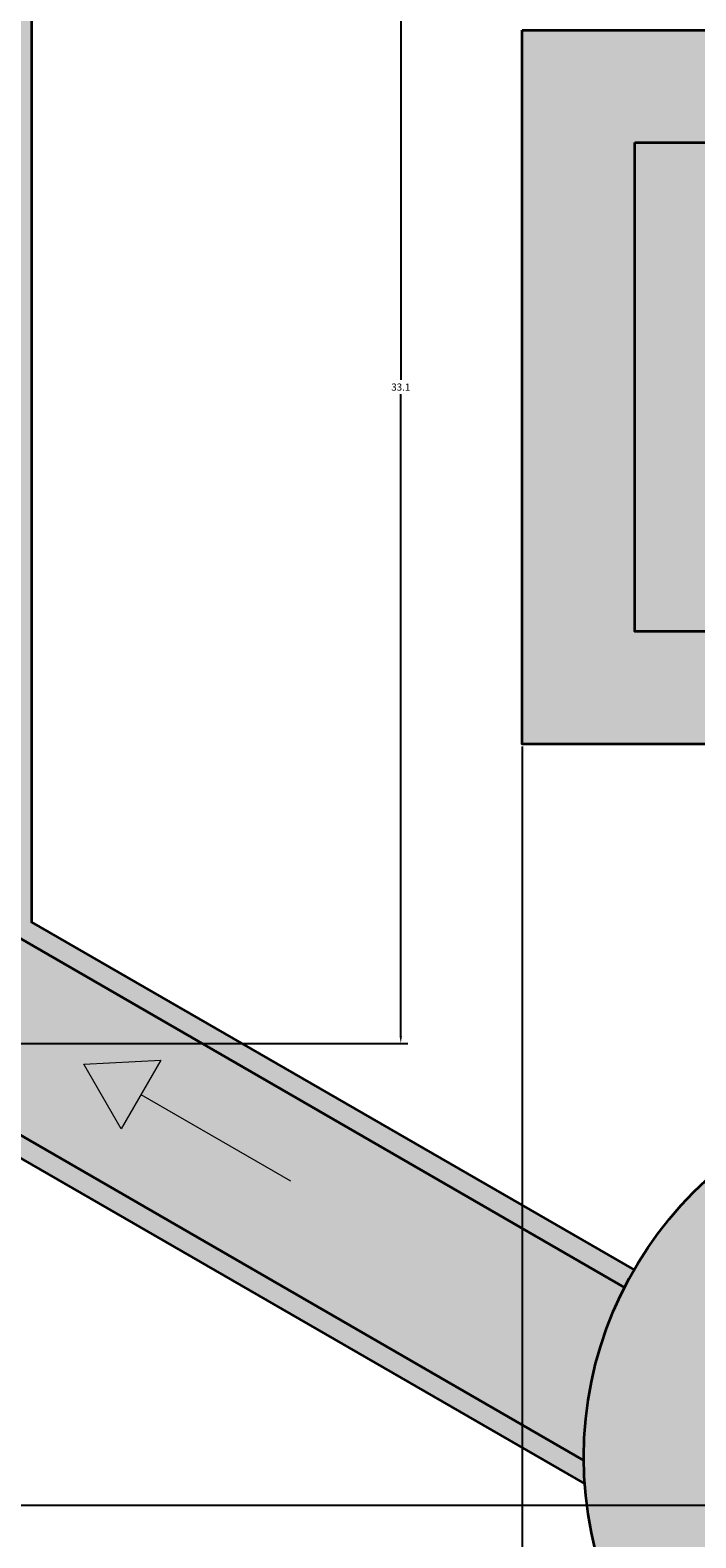
# Model space of a CAD drawing. Units: inches. Extents: x -1 to 292, y -3 to 199.
# Tile 43 of 52: x 220 to 237, y 43 to 81. Entities that reach past the tile are written whole.
import ezdxf

# ---------------------------------------------------------------- set-up
doc = ezdxf.new("R2010")
doc.units = ezdxf.units.IN
doc.header["$MEASUREMENT"] = 0
for name, color, linetype, lineweight in [('M-ANNO-SYMB', 1, 'Continuous', 18), ('M-DIMS', 2, 'Continuous', 18), ('M-EQPM', 7, 'Continuous', 35), ('M-PATT', 8, 'Continuous', 13)]:
    doc.layers.add(name, color=color, linetype=linetype, lineweight=lineweight)
doc.styles.get("Standard").update_dxf_attribs({"font": 'arial.ttf'})
doc.dimstyles.get("Standard").update_dxf_attribs({"dimtxt": 0.18, "dimasz": 0.18, "dimexe": 0.18, "dimexo": 0.0625, "dimgap": 0.09, "dimtad": 0, "dimtih": 1, "dimtoh": 1, "dimdec": 4, "dimzin": 0, "dimdsep": 46, "dimtxsty": 'Standard', "dimcen": 0.09, "dimadec": 0, "dimazin": 0, "dimtfac": 1, "dimtdec": 4, "dimtofl": 0, "dimtmove": 0, "dimatfit": 3, "dimfxl": 1, "dimtolj": 1, "dimtzin": 0, "dimarcsym": 0})

# ---------------------------------------------------------------- blocks, each defined once
blk = doc.blocks.new('FLOW-ARROW-WATER')
blk.add_line((223.29, 53.741), (227.063, 51.564))
blk.add_lwpolyline([(222.79, 52.875), (221.849, 54.506), (223.79, 54.608)], close=True)
blk = doc.blocks.new('*D10')
at = {"layer": 'Defpoints', "color": 0, "transparency": 16777216}
for p in [(169.176, 99.774), (169.176, 43.391), (292.04, 43.391)]:
    blk.add_point(p, dxfattribs=at)
at = {"layer": 'M-DIMS', "color": 0, "lineweight": -2, "transparency": 16777216}
for p, q in [((169.239, 99.774), (292.22, 99.774)), ((292.04, 99.594), (292.04, 71.764)), ((292.04, 43.571), (292.04, 71.4)), ((169.239, 43.391), (292.22, 43.391))]:
    blk.add_line(p, q, dxfattribs=at)
at = {"layer": 'M-DIMS', "color": 0, "transparency": 16777216}
for points in [[(292.01, 99.594), (292.07, 99.594), (292.04, 99.774)], [(292.01, 43.571), (292.07, 43.571), (292.04, 43.391)]]:
    blk.add_solid(points, dxfattribs=at)
at = {"layer": 'M-DIMS', "color": 0, "transparency": 16777216, "insert": (292.04, 71.582), "char_height": 0.18, "attachment_point": 5}
blk.add_mtext('\\A1;56.38', dxfattribs=at)
blk = doc.blocks.new('*D25')
at = {"layer": 'Defpoints', "color": 0, "transparency": 16777216}
for p in [(273.066, 88.419), (215.241, 88.13), (273.066, -2.71)]:
    blk.add_point(p, dxfattribs=at)
at = {"layer": 'M-DIMS', "color": 0, "lineweight": -2, "transparency": 16777216}
for p, q in [((273.066, 88.357), (273.066, -2.89)), ((215.241, 88.068), (215.241, -2.89)), ((215.421, -2.71), (243.76, -2.71)), ((272.886, -2.71), (244.547, -2.71))]:
    blk.add_line(p, q, dxfattribs=at)
at = {"layer": 'M-DIMS', "color": 0, "transparency": 16777216}
for points in [[(215.421, -2.68), (215.421, -2.74), (215.241, -2.71)], [(272.886, -2.68), (272.886, -2.74), (273.066, -2.71)]]:
    blk.add_solid(points, dxfattribs=at)
at = {"layer": 'M-DIMS', "color": 0, "transparency": 16777216, "insert": (244.153, -2.71), "char_height": 0.18, "attachment_point": 5}
blk.add_mtext('\\A1;57.83', dxfattribs=at)
blk = doc.blocks.new('*D26')
at = {"layer": 'Defpoints', "color": 0, "transparency": 16777216}
for p in [(215.241, 88.13), (215.241, 55.034), (229.841, 55.034)]:
    blk.add_point(p, dxfattribs=at)
at = {"layer": 'M-DIMS', "color": 0, "lineweight": -2, "transparency": 16777216}
for p, q in [((215.303, 88.13), (230.021, 88.13)), ((229.841, 87.95), (229.841, 71.764)), ((229.841, 55.214), (229.841, 71.4)), ((215.303, 55.034), (230.021, 55.034))]:
    blk.add_line(p, q, dxfattribs=at)
at = {"layer": 'M-DIMS', "color": 0, "transparency": 16777216}
for points in [[(229.811, 87.95), (229.871, 87.95), (229.841, 88.13)], [(229.811, 55.214), (229.871, 55.214), (229.841, 55.034)]]:
    blk.add_solid(points, dxfattribs=at)
at = {"layer": 'M-DIMS', "color": 0, "transparency": 16777216, "insert": (229.841, 71.582), "char_height": 0.18, "attachment_point": 5}
blk.add_mtext('\\A1;33.1', dxfattribs=at)
blk = doc.blocks.new('*D30')
at = {"layer": 'Defpoints', "color": 0, "transparency": 16777216}
for p in [(232.903, 62.582), (254.903, 62.582), (254.903, -2.71)]:
    blk.add_point(p, dxfattribs=at)
at = {"layer": 'M-DIMS', "color": 0, "lineweight": -2, "transparency": 16777216}
for p, q in [((232.903, 62.52), (232.903, -2.89)), ((254.903, 62.52), (254.903, -2.89)), ((233.083, -2.71), (243.684, -2.71)), ((254.723, -2.71), (244.123, -2.71))]:
    blk.add_line(p, q, dxfattribs=at)
at = {"layer": 'M-DIMS', "color": 0, "transparency": 16777216}
for points in [[(233.083, -2.68), (233.083, -2.74), (232.903, -2.71)], [(254.723, -2.68), (254.723, -2.74), (254.903, -2.71)]]:
    blk.add_solid(points, dxfattribs=at)
at = {"layer": 'M-DIMS', "color": 0, "transparency": 16777216, "insert": (243.903, -2.71), "char_height": 0.18, "attachment_point": 5}
blk.add_mtext('\\A1;22', dxfattribs=at)
blk = doc.blocks.new('*D36')
at = {"layer": 'Defpoints', "color": 0, "transparency": 16777216}
for p in [(234.455, 44.597), (253.352, 44.598)]:
    blk.add_point(p, dxfattribs=at)
at = {"layer": 'M-DIMS', "color": 0, "lineweight": -2, "transparency": 16777216}
for p, q in [((243.813, 44.598), (243.993, 44.598)), ((243.903, 44.508), (243.903, 44.688)), ((259.021, 44.598), (253.532, 44.598))]:
    blk.add_line(p, q, dxfattribs=at)
at = {"layer": 'M-DIMS', "color": 0, "transparency": 16777216}
blk.add_solid([(253.532, 44.628), (253.532, 44.568), (253.352, 44.598)], dxfattribs=at)
at = {"layer": 'M-DIMS', "color": 0, "transparency": 16777216, "insert": (259.582, 44.598), "char_height": 0.18, "attachment_point": 5}
blk.add_mtext('\\A1;∅18.897', dxfattribs=at)

msp = doc.modelspace()

# ---------------------------------------------------------------- hatches: boundary and pattern name
at = {"layer": 'M-PATT'}
h = msp.add_hatch(color=256, dxfattribs=at)
h.set_gradient(color1=(0, 255, 255), color2=(0, 255, 255), tint=1, name='CYLINDER')
h.paths.add_polyline_path([(256.8092, 99.5764), (256.4077, 99.3157), (253.7155, 100.87), (251.3221, 99.3157), (248.6299, 100.87), (246.2365, 99.3157), (243.5443, 100.87), (241.1509, 99.3157), (238.4587, 100.87), (236.4209, 99.5466), (236.4209, 97.1861), (234.9209, 97.1861), (234.9209, 99.9764), (233.3731, 100.87), (230.9797, 99.3157, 1.0704128)])
h.paths.add_polyline_path([(234.4549, 44.5975, 1), (253.3518, 44.5975, 1)])
h.paths.add_polyline_path([(235.4822, 48.8821), (220.034, 57.8011), (220.034, 85.363), (232.4507, 92.5318, -0.0853739), (231.0925, 96.7051), (215.7407, 87.8418), (215.7407, 55.3224), (234.4552, 44.5176, -0.0021162), (234.4549, 44.5975, -0.1182098)])
h.paths.add_polyline_path([(222.7904, 52.8755), (221.8492, 54.5058), (223.7904, 54.6075)], flags=16)
h.paths.add_polyline_path([(216.828, 66.8912), (217.7692, 68.5216), (218.828, 66.8912)], flags=16)
h.paths.add_polyline_path([(216.8084, 83.826), (217.7497, 85.4564), (218.8084, 83.826)], flags=16)
h.paths.add_polyline_path([(226.468, 92.8803), (228.3442, 93.0348), (227.6068, 91.2362)], flags=16)
h.paths.add_polyline_path([(272.5659, 88.1304), (260.2765, 95.2257), (259.0113, 93.0196), (263.0639, 91.1046), (263.4912, 92.0087), (264.5631, 90.4612), (262.6367, 90.2004), (263.0639, 91.1046), (259.0113, 93.0196), (257.8918, 91.0677), (267.7726, 85.363), (267.7726, 57.8011), (255.5043, 50.718), (257.0663, 46.085), (272.5659, 55.0337)])
h.paths.add_polyline_path([(263.6286, 51.5636), (261.7461, 51.5636), (262.6286, 53.2956)], flags=16)
h.paths.add_polyline_path([(269.8773, 65.3608), (268.8186, 66.9911), (270.8186, 66.9911)], flags=16)
h.paths.add_polyline_path([(269.8773, 80.8843), (268.8186, 82.5146), (270.8186, 82.5146)], flags=16)
h.paths.add_polyline_path([(255.5043, 50.718), (252.3244, 48.8821, -0.1182098), (253.3518, 44.5975, -0.0177685), (253.3279, 43.9266), (257.0663, 46.085)])
h.paths.add_polyline_path([(260.2765, 95.2257), (256.7809, 97.2439, -0.0959457), (255.356, 92.5318), (257.8918, 91.0677)])
h = msp.add_hatch(color=256, dxfattribs=at)
h.set_gradient(color1=(76, 38, 47), color2=(76, 38, 47), tint=1, name='CYLINDER')
h.paths.add_polyline_path([(267.2726, 58.0898), (255.3414, 51.2013), (255.5043, 50.718), (267.7726, 57.8011), (267.7726, 85.363), (257.8918, 91.0677), (257.643, 90.634), (267.2726, 85.0743)])
h.paths.add_polyline_path([(272.5659, 55.0337), (257.0663, 46.085), (257.2293, 45.6017), (273.0659, 54.745), (273.0659, 88.4191), (260.5253, 95.6595), (260.2765, 95.2257), (272.5659, 88.1304)])
h.paths.add_polyline_path([(215.2407, 55.0337), (234.4787, 43.9266, -0.0156517), (234.4552, 44.5176), (215.7407, 55.3224), (215.7407, 87.8418), (231.0925, 96.7051, -0.0104859), (231.0257, 97.2439), (215.2407, 88.1304)])
h.paths.add_polyline_path([(220.034, 57.8011), (235.4822, 48.8821, -0.0132367), (235.7207, 49.3218), (220.534, 58.0898), (220.534, 85.0743), (232.6923, 92.0939, -0.0096587), (232.4507, 92.5318), (220.034, 85.363)])
h = msp.add_hatch(color=256, dxfattribs=at)
h.set_gradient(color1=(0, 0, 255), color2=(0, 0, 255), tint=1, name='CYLINDER')
h.paths.add_polyline_path([(227.6068, 91.2362), (228.3442, 93.0348), (226.468, 92.8803)])
h.paths.add_polyline_path([(218.8084, 83.826), (217.7497, 85.4564), (216.8084, 83.826)])
h.paths.add_polyline_path([(262.6367, 90.2004), (264.5631, 90.4612), (263.4912, 92.0087)])
h.paths.add_polyline_path([(217.7692, 68.5216), (216.828, 66.8912), (218.828, 66.8912)])
h.paths.add_polyline_path([(223.7904, 54.6075), (221.8492, 54.5058), (222.7904, 52.8755)])
h.paths.add_polyline_path([(262.6286, 53.2956), (261.7461, 51.5636), (263.6286, 51.5636)])
h.paths.add_polyline_path([(268.8186, 82.5146), (269.8773, 80.8843), (270.8186, 82.5146)])
h.paths.add_polyline_path([(268.8186, 66.9911), (269.8773, 65.3608), (270.8186, 66.9911)])
h = msp.add_hatch(color=256, dxfattribs=at)
h.set_gradient(color1=(242, 103, 34), color2=(242, 103, 34), tint=1, name='CYLINDER')
h.paths.add_polyline_path([(232.9033, 62.5821), (254.9033, 62.5821), (254.9033, 80.5821), (251.8779, 80.5821), (250.2521, 77.7473), (252.0686, 77.7473), (252.0686, 65.4168), (235.7381, 65.4168), (235.7381, 77.7473), (250.2521, 77.7473), (251.8779, 80.5821), (232.9033, 80.5821)])
h = msp.add_hatch(color=256, dxfattribs=at)
h.set_gradient(color1=(76, 38, 47), color2=(76, 38, 47), tint=1, name='CYLINDER')
h.paths.add_polyline_path([(237.744, 67.4228), (237.744, 75.7414), (249.1016, 75.7414), (250.2521, 77.7473), (235.7381, 77.7473), (235.7381, 65.4168), (252.0686, 65.4168), (252.0686, 77.7473), (250.2521, 77.7473), (249.1016, 75.7414), (250.0626, 75.7414), (250.0626, 67.4228)])

# ---------------------------------------------------------------- linework, layer by layer
at = {"layer": 'M-EQPM'}
for points in [[(231.0257, 97.2439), (215.2407, 88.1304), (215.2407, 55.0337), (234.4787, 43.9266)], [(231.0925, 96.7051), (215.7407, 87.8418), (215.7407, 55.3224), (234.4552, 44.5176)], [(232.4507, 92.5318), (220.034, 85.363), (220.034, 57.8011), (235.4822, 48.8821)], [(232.6923, 92.0939), (220.534, 85.0743), (220.534, 58.0898), (235.7207, 49.3218)]]:
    msp.add_lwpolyline(points, dxfattribs=at)
for points in [[(232.9033, 80.5821), (254.9033, 80.5821), (254.9033, 62.5821), (232.9033, 62.5821)], [(235.7381, 77.7473), (252.0686, 77.7473), (252.0686, 65.4168), (235.7381, 65.4168)]]:
    msp.add_lwpolyline(points, close=True, dxfattribs=at)
msp.add_circle((243.9033, 44.5975), 9.4484, dxfattribs=at)

# ---------------------------------------------------------------- block references
at = {"layer": 'M-ANNO-SYMB'}
msp.add_blockref('FLOW-ARROW-WATER', (0, 0), dxfattribs=at)

# ---------------------------------------------------------------- dimensions: what is measured, and where the dimension line sits
at = {"layer": 'M-DIMS'}
for base, p1, p2, angle, override, picture, middle in [((292.0399, 43.3906), (169.176, 99.7735), (169.176, 43.3906), 90, {"dimdec": 2, "dimlfac": 1, "dimrnd": 0, "dimzin": 0, "dimdsep": 46, "dimlunit": 2}, '*D10', (292.0399, 71.5821)), ((229.8407, 55.0337), (215.2407, 88.1304), (215.2407, 55.0337), 270, {"dimdec": 1, "dimlfac": 1, "dimrnd": 0, "dimzin": 0, "dimdsep": 46, "dimlunit": 2}, '*D26', (229.8407, 71.5821))]:
    dim = msp.add_linear_dim(base=base, p1=p1, p2=p2, angle=angle, dimstyle='Standard', override=override, dxfattribs=at)
    dim.commit()
    dim.dimension.update_dxf_attribs({"geometry": picture, "text_midpoint": middle})
for base, p1, p2, override, picture, middle in [((273.0659, -2.7104), (215.2407, 88.1304), (273.0659, 88.4191), {"dimdec": 2, "dimlfac": 1, "dimrnd": 0, "dimzin": 0, "dimdsep": 46, "dimlunit": 2}, '*D25', (244.1533, -2.7104)), ((254.9033, -2.7104), (232.9033, 62.5821), (254.9033, 62.5821), {"dimdec": 0, "dimlfac": 1, "dimrnd": 0, "dimzin": 0, "dimdsep": 46, "dimlunit": 2}, '*D30', (243.9033, -2.7104))]:
    dim = msp.add_linear_dim(base=base, p1=p1, p2=p2, dimstyle='Standard', override=override, dxfattribs=at)
    dim.commit()
    dim.dimension.update_dxf_attribs({"geometry": picture, "text_midpoint": middle})
dim = msp.add_diameter_dim_2p(p1=(234.4549, 44.5971), p2=(253.3518, 44.598), dimstyle='Standard', override={"dimdec": 3, "dimlfac": 1, "dimrnd": 0, "dimzin": 0, "dimdsep": 46, "dimlunit": 2}, dxfattribs=at)
dim.commit()
dim.dimension.update_dxf_attribs({"geometry": '*D36', "text_midpoint": (259.0208, 44.5983), "dimtype": 163})

doc.saveas('drawing.dxf')
